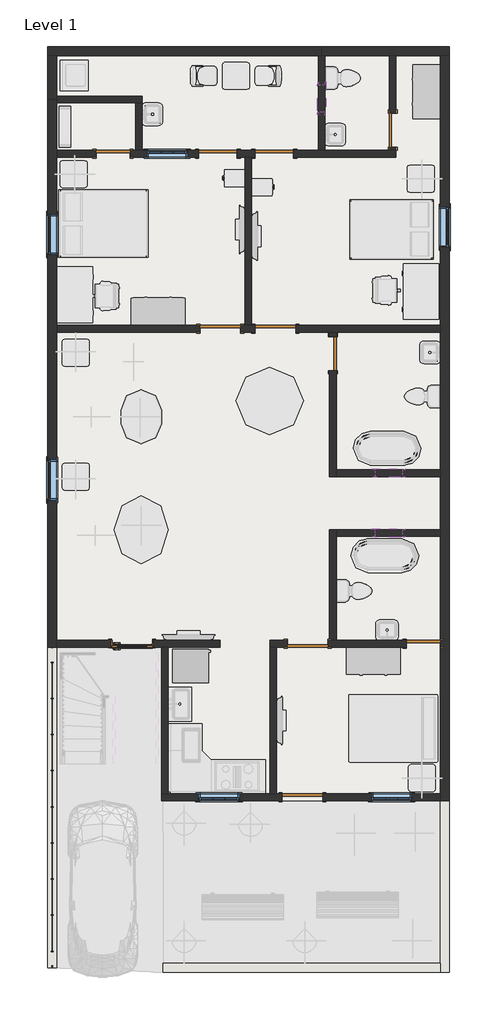
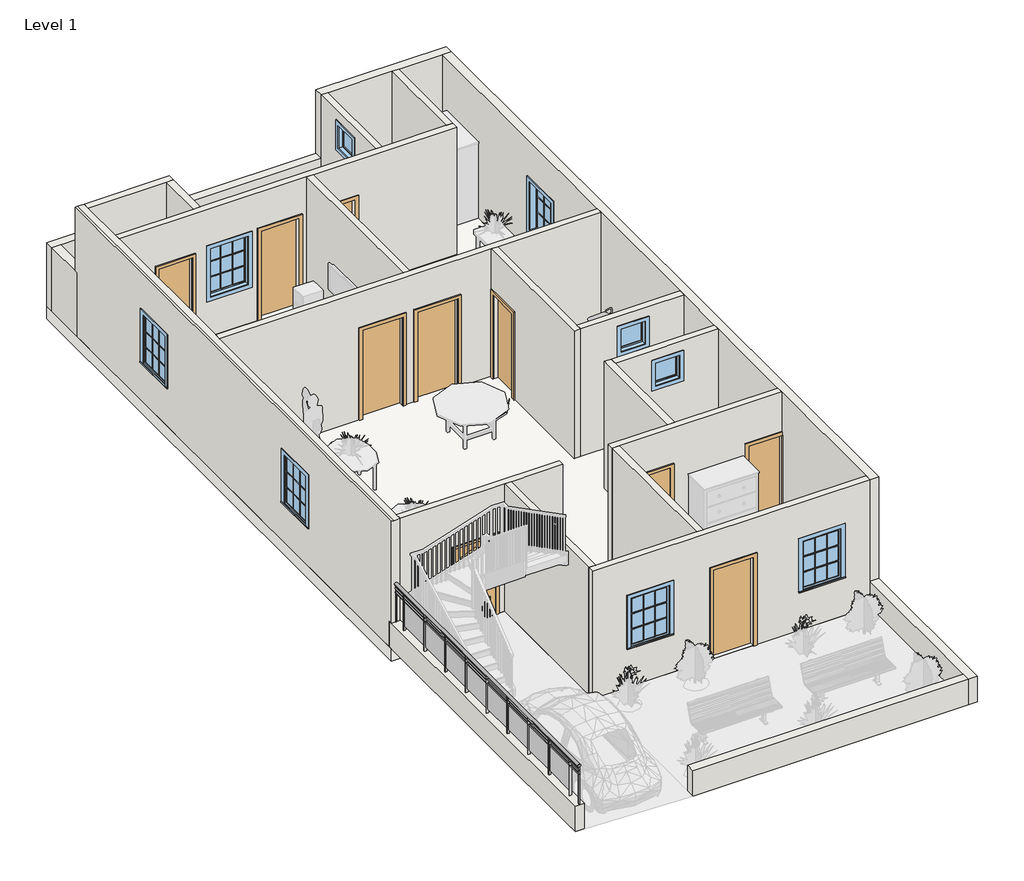
# One storey, part 1 of 3: 24 walls, 11 doors, 9 windows, 1 railing, 1 slab.
"""IFC4 building model written with IfcOpenShell, lengths in millimetres."""

from ifc_helpers import new_model, si_unit, point, frame, origin, origin_with_axes, place, context, project, spatial, polyline, ellipse_curve, trimmed, outline, extrude, faceted_brep, transform, mapped, element, save
from ifc_brep_helpers import plane_surface, extruded_surface, advanced_brep
from components import door_6e7732ad, door_059fdd7e, door_255cab33, door_b6e9fca3, door_99d96fc5, door_16372e1c, door_686f89d2, window_5c190c7e, window_29c06734, window_3d781103

model = new_model("IFC4")

# Units and contexts
model_context = context("Model", 3, world=origin())
ifc_project = project(units=[si_unit("LENGTHUNIT", "METRE", prefix="MILLI")], contexts=[model_context])

# Site, building, storey
site = spatial("IfcSite", under=ifc_project)
building = spatial("IfcBuilding", under=site)
storey = spatial("IfcBuildingStorey", under=building, Name="Level 1", Elevation=0.0)

# Doors
placement = place(None, origin())
door_shape = door_6e7732ad(model_context)
element("IfcDoor", 1, ObjectType="36\" x 74\"", at=placement, inside=storey, context=model_context, shape_type="MappedRepresentation", body=[
    mapped(door_shape, transform((-11373.4589543, -1136.727182, 0.0), x_axis=(-1.0, 0.0, 0.0), y_axis=(0.0, -1.0, 0.0), z_axis=(0.0, 0.0, 1.0))),
])
door_2_shape = door_059fdd7e(model_context)
element("IfcDoor", 2, ObjectType="Single-Flush : 30\" x 80\"", at=placement, inside=storey, context=model_context, shape_type="MappedRepresentation", body=[
    mapped(door_2_shape, transform((-11805.2589543, 9890.047818, 0.0), x_axis=(1.0, 0.0, 0.0), y_axis=(0.0, 1.0, 0.0), z_axis=(0.0, 0.0, 1.0))),
])
element("IfcDoor", 3, ObjectType="Single-Flush : 30\" x 80\"", at=placement, inside=storey, context=model_context, shape_type="MappedRepresentation", body=[
    mapped(door_2_shape, transform((-4820.2589543, -1133.552182, 0.0), x_axis=(1.0, 0.0, 0.0), y_axis=(0.0, 1.0, 0.0), z_axis=(0.0, 0.0, 1.0))),
])
door_3_shape = door_255cab33(model_context)
element("IfcDoor", 4, ObjectType="Single-Flush : 30\" x 80\"", at=placement, inside=storey, context=model_context, shape_type="MappedRepresentation", body=[
    mapped(door_3_shape, transform((-5506.0589543, 10423.447818, 0.0), x_axis=(0.0, -1.0, 0.0), y_axis=(1.0, 0.0, 0.0), z_axis=(0.0, 0.0, 1.0))),
])
element("IfcDoor", 5, ObjectType="Single-Flush : 30\" x 80\"", at=placement, inside=storey, context=model_context, shape_type="MappedRepresentation", body=[
    mapped(door_3_shape, transform((-6852.2589543, 5394.247818, 0.0), x_axis=(0.0, 1.0, 0.0), y_axis=(-1.0, 0.0, 0.0), z_axis=(0.0, 0.0, 1.0))),
])
door_4_shape = door_b6e9fca3(model_context)
element("IfcDoor", 6, ObjectType="Single-Flush : 34\" x 84\"", at=placement, inside=storey, context=model_context, shape_type="MappedRepresentation", body=[
    mapped(door_4_shape, transform((-9443.0589543, 9890.047818, 0.0), x_axis=(1.0, 0.0, 0.0), y_axis=(0.0, 1.0, 0.0), z_axis=(0.0, 0.0, 1.0))),
])
door_5_shape = door_99d96fc5(model_context)
element("IfcDoor", 7, ObjectType="Single-Flush : 34\" x 84\"", at=placement, inside=storey, context=model_context, shape_type="MappedRepresentation", body=[
    mapped(door_5_shape, transform((-8173.0589543, 9890.047818, 0.0), x_axis=(-1.0, 0.0, 0.0), y_axis=(0.0, -1.0, 0.0), z_axis=(0.0, 0.0, 1.0))),
])
door_6_shape = door_16372e1c(model_context)
element("IfcDoor", 8, ObjectType="Single-Flush : 36\" x 84\"", at=placement, inside=storey, context=model_context, shape_type="MappedRepresentation", body=[
    mapped(door_6_shape, transform((-9392.2589543, 5953.047818, 0.0), x_axis=(1.0, 0.0, 0.0), y_axis=(0.0, 1.0, 0.0), z_axis=(0.0, 0.0, 1.0))),
])
element("IfcDoor", 9, ObjectType="Single-Flush : 36\" x 84\"", at=placement, inside=storey, context=model_context, shape_type="MappedRepresentation", body=[
    mapped(door_6_shape, transform((-7423.7589543, -1133.552182, 0.0), x_axis=(-1.0, 0.0, 0.0), y_axis=(0.0, -1.0, 0.0), z_axis=(0.0, 0.0, 1.0))),
])
door_7_shape = door_686f89d2(model_context)
element("IfcDoor", 10, ObjectType="Single-Flush : 36\" x 84\"", at=placement, inside=storey, context=model_context, shape_type="MappedRepresentation", body=[
    mapped(door_7_shape, transform((-8147.6589543, 5953.047818, 0.0), x_axis=(-1.0, 0.0, 0.0), y_axis=(0.0, -1.0, 0.0), z_axis=(0.0, 0.0, 1.0))),
])
element("IfcDoor", 11, ObjectType="Single-Flush : 36\" x 84\"", at=placement, inside=storey, context=model_context, shape_type="MappedRepresentation", body=[
    mapped(door_7_shape, transform((-7538.0589543, -4587.952182, 0.0), x_axis=(-1.0, 0.0, 0.0), y_axis=(0.0, -1.0, 0.0), z_axis=(0.0, 0.0, 1.0))),
])

# Railing
element("IfcRailing", 12, ObjectType="Glass Panel - Bottom Fill", at=placement, inside=storey, context=model_context, shape_type="SolidModel", body=[
    advanced_brep(
    [(-13138.7589543, -1209.752182, 1524.0), (-13214.9589543, -1209.752182, 1524.0), (-13138.7589543, -8397.952182, 1524.0), (-13214.9589543, -8397.952182, 1524.0)],
    [
        (0, 1, ellipse_curve(frame((-13176.8589543, -1209.752182, 1524.0), z_axis=(0.0, 1.0, 0.0), x_axis=(-1.0, 0.0, 0.0)), 38.1, 28.575)),
        (1, 0, ellipse_curve(frame((-13176.8589543, -1209.752182, 1524.0), z_axis=(0.0, 1.0, 0.0), x_axis=(-1.0, 0.0, 0.0)), 38.1, 28.575)),
        (2, 3, ellipse_curve(frame((-13176.8589543, -8397.952182, 1524.0), z_axis=(0.0, -1.0, 0.0), x_axis=(-1.0, 0.0, 0.0)), 38.1, 28.575)),
        (3, 2, ellipse_curve(frame((-13176.8589543, -8397.952182, 1524.0), z_axis=(0.0, -1.0, 0.0), x_axis=(-1.0, 0.0, 0.0)), 38.1, 28.575)),
        (0, 2),
        (3, 1),
    ],
    [
        plane_surface(frame((-13176.8589543, -1209.752182, 1524.0), z_axis=(0.0, 1.0, 0.0), x_axis=(0.0, 0.0, -1.0))),
        plane_surface(frame((-13176.8589543, -8397.952182, 1524.0), z_axis=(0.0, -1.0, 0.0), x_axis=(0.0, 0.0, -1.0))),
        extruded_surface(trimmed(ellipse_curve(frame((-13176.8589543, -8397.952182, 1524.0), z_axis=(0.0, 1.0, 0.0), x_axis=(-1.0, 0.0, 0.0)), 38.1, 28.575), [point((-13138.7589543, -8397.952182, 1524.0))], [point((-13214.9589543, -8397.952182, 1524.0))], True, "CARTESIAN"), (0.0, 7188.200000000001, 0.0), 7188.200000000001),
        extruded_surface(trimmed(ellipse_curve(frame((-13176.8589543, -8397.952182, 1524.0), z_axis=(0.0, 1.0, 0.0), x_axis=(-1.0, 0.0, 0.0)), 38.1, 28.575), [point((-13214.9589543, -8397.952182, 1524.0))], [point((-13138.7589543, -8397.952182, 1524.0))], True, "CARTESIAN"), (0.0, 7188.200000000001, 0.0), 7188.200000000001),
    ],
    [
        (0, [[1, 2]]),
        (1, [[3, 4]]),
        (2, [[-1, 5, -4, 6]]),
        (3, [[-2, -6, -3, -5]]),
    ],
),
    extrude(outline(polyline([(-13189.5589543, -1209.752182), (-13164.1589543, -1209.752182), (-13164.1589543, -8397.952182), (-13189.5589543, -8397.952182), (-13189.5589543, -1209.752182)])), frame((0.0, 0.0, 1409.7), z_axis=(0.0, 0.0, 1.0), x_axis=(1.0, 0.0, 0.0)), (0.0, 0.0, 1.0), 25.4),
    extrude(outline(polyline([(-13189.5589543, -1209.752182), (-13164.1589543, -1209.752182), (-13164.1589543, -8397.952182), (-13189.5589543, -8397.952182), (-13189.5589543, -1209.752182)])), frame((0.0, 0.0, 1308.1), z_axis=(0.0, 0.0, 1.0), x_axis=(1.0, 0.0, 0.0)), (0.0, 0.0, 1.0), 25.4),
    extrude(outline(polyline([(-13202.2589543, -8048.702182), (-13151.4589543, -8048.702182), (-13151.4589543, -8061.402182), (-13202.2589543, -8061.402182), (-13202.2589543, -8048.702182)])), frame((0.0, 0.0, 609.6), z_axis=(0.0, 0.0, 1.0), x_axis=(1.0, 0.0, 0.0)), (0.0, 0.0, 1.0), 885.6788223),
    extrude(outline(polyline([(-13170.3237973, -7242.252182), (-13170.3237973, -8055.052182), (-13176.6737973, -8055.052182), (-13176.6737973, -7242.252182), (-13170.3237973, -7242.252182)])), frame((0.0, 0.0, 711.2), z_axis=(0.0, 0.0, 1.0), x_axis=(1.0, 0.0, 0.0)), (0.0, 0.0, 1.0), 596.9),
    extrude(outline(polyline([(-13202.2589543, -7235.902182), (-13151.4589543, -7235.902182), (-13151.4589543, -7248.602182), (-13202.2589543, -7248.602182), (-13202.2589543, -7235.902182)])), frame((0.0, 0.0, 609.6), z_axis=(0.0, 0.0, 1.0), x_axis=(1.0, 0.0, 0.0)), (0.0, 0.0, 1.0), 885.6788223),
    extrude(outline(polyline([(-13170.3237973, -6429.452182), (-13170.3237973, -7242.252182), (-13176.6737973, -7242.252182), (-13176.6737973, -6429.452182), (-13170.3237973, -6429.452182)])), frame((0.0, 0.0, 711.2), z_axis=(0.0, 0.0, 1.0), x_axis=(1.0, 0.0, 0.0)), (0.0, 0.0, 1.0), 596.9),
    extrude(outline(polyline([(-13202.2589543, -6423.102182), (-13151.4589543, -6423.102182), (-13151.4589543, -6435.802182), (-13202.2589543, -6435.802182), (-13202.2589543, -6423.102182)])), frame((0.0, 0.0, 609.6), z_axis=(0.0, 0.0, 1.0), x_axis=(1.0, 0.0, 0.0)), (0.0, 0.0, 1.0), 885.6788223),
    extrude(outline(polyline([(-13170.3237973, -5616.652182), (-13170.3237973, -6429.452182), (-13176.6737973, -6429.452182), (-13176.6737973, -5616.652182), (-13170.3237973, -5616.652182)])), frame((0.0, 0.0, 711.2), z_axis=(0.0, 0.0, 1.0), x_axis=(1.0, 0.0, 0.0)), (0.0, 0.0, 1.0), 596.9),
    extrude(outline(polyline([(-13202.2589543, -5610.302182), (-13151.4589543, -5610.302182), (-13151.4589543, -5623.002182), (-13202.2589543, -5623.002182), (-13202.2589543, -5610.302182)])), frame((0.0, 0.0, 609.6), z_axis=(0.0, 0.0, 1.0), x_axis=(1.0, 0.0, 0.0)), (0.0, 0.0, 1.0), 885.6788223),
    extrude(outline(polyline([(-13170.3237973, -4803.852182), (-13170.3237973, -5616.652182), (-13176.6737973, -5616.652182), (-13176.6737973, -4803.852182), (-13170.3237973, -4803.852182)])), frame((0.0, 0.0, 711.2), z_axis=(0.0, 0.0, 1.0), x_axis=(1.0, 0.0, 0.0)), (0.0, 0.0, 1.0), 596.9),
    extrude(outline(polyline([(-13202.2589543, -4797.502182), (-13151.4589543, -4797.502182), (-13151.4589543, -4810.202182), (-13202.2589543, -4810.202182), (-13202.2589543, -4797.502182)])), frame((0.0, 0.0, 609.6), z_axis=(0.0, 0.0, 1.0), x_axis=(1.0, 0.0, 0.0)), (0.0, 0.0, 1.0), 885.6788223),
    extrude(outline(polyline([(-13170.3237973, -3991.052182), (-13170.3237973, -4803.852182), (-13176.6737973, -4803.852182), (-13176.6737973, -3991.052182), (-13170.3237973, -3991.052182)])), frame((0.0, 0.0, 711.2), z_axis=(0.0, 0.0, 1.0), x_axis=(1.0, 0.0, 0.0)), (0.0, 0.0, 1.0), 596.9),
    extrude(outline(polyline([(-13202.2589543, -3984.702182), (-13151.4589543, -3984.702182), (-13151.4589543, -3997.402182), (-13202.2589543, -3997.402182), (-13202.2589543, -3984.702182)])), frame((0.0, 0.0, 609.6), z_axis=(0.0, 0.0, 1.0), x_axis=(1.0, 0.0, 0.0)), (0.0, 0.0, 1.0), 885.6788223),
    extrude(outline(polyline([(-13170.3237973, -3178.252182), (-13170.3237973, -3991.052182), (-13176.6737973, -3991.052182), (-13176.6737973, -3178.252182), (-13170.3237973, -3178.252182)])), frame((0.0, 0.0, 711.2), z_axis=(0.0, 0.0, 1.0), x_axis=(1.0, 0.0, 0.0)), (0.0, 0.0, 1.0), 596.9),
    extrude(outline(polyline([(-13202.2589543, -3171.902182), (-13151.4589543, -3171.902182), (-13151.4589543, -3184.602182), (-13202.2589543, -3184.602182), (-13202.2589543, -3171.902182)])), frame((0.0, 0.0, 609.6), z_axis=(0.0, 0.0, 1.0), x_axis=(1.0, 0.0, 0.0)), (0.0, 0.0, 1.0), 885.6788223),
    extrude(outline(polyline([(-13170.3237973, -2365.452182), (-13170.3237973, -3178.252182), (-13176.6737973, -3178.252182), (-13176.6737973, -2365.452182), (-13170.3237973, -2365.452182)])), frame((0.0, 0.0, 711.2), z_axis=(0.0, 0.0, 1.0), x_axis=(1.0, 0.0, 0.0)), (0.0, 0.0, 1.0), 596.9),
    extrude(outline(polyline([(-13202.2589543, -2359.102182), (-13151.4589543, -2359.102182), (-13151.4589543, -2371.802182), (-13202.2589543, -2371.802182), (-13202.2589543, -2359.102182)])), frame((0.0, 0.0, 609.6), z_axis=(0.0, 0.0, 1.0), x_axis=(1.0, 0.0, 0.0)), (0.0, 0.0, 1.0), 885.6788223),
    extrude(outline(polyline([(-13170.3237973, -1552.652182), (-13170.3237973, -2365.452182), (-13176.6737973, -2365.452182), (-13176.6737973, -1552.652182), (-13170.3237973, -1552.652182)])), frame((0.0, 0.0, 711.2), z_axis=(0.0, 0.0, 1.0), x_axis=(1.0, 0.0, 0.0)), (0.0, 0.0, 1.0), 596.9),
    extrude(outline(polyline([(-13202.2589543, -1546.302182), (-13151.4589543, -1546.302182), (-13151.4589543, -1559.002182), (-13202.2589543, -1559.002182), (-13202.2589543, -1546.302182)])), frame((0.0, 0.0, 609.6), z_axis=(0.0, 0.0, 1.0), x_axis=(1.0, 0.0, 0.0)), (0.0, 0.0, 1.0), 885.6788223),
    extrude(outline(polyline([(-13186.3839543, -8385.252182), (-13167.3339543, -8385.252182), (-13167.3339543, -8404.302182), (-13186.3839543, -8404.302182), (-13186.3839543, -8385.252182)])), frame((0.0, 0.0, 609.6), z_axis=(0.0, 0.0, 1.0), x_axis=(1.0, 0.0, 0.0)), (0.0, 0.0, 1.0), 885.6788223),
    extrude(outline(polyline([(-13186.3839543, -1203.402182), (-13167.3339543, -1203.402182), (-13167.3339543, -1222.452182), (-13186.3839543, -1222.452182), (-13186.3839543, -1203.402182)])), frame((0.0, 0.0, 609.6), z_axis=(0.0, 0.0, 1.0), x_axis=(1.0, 0.0, 0.0)), (0.0, 0.0, 1.0), 885.6788223),
])

# Slab
element("IfcSlab", 13, ObjectType="Generic - 12\"", at=placement, inside=storey, context=model_context, shape_type="SweptSolid", body=[
    extrude(outline(polyline([(-4236.0589543, 12303.047818), (-4236.0589543, -4664.152182), (-10713.0589543, -4664.152182), (-10713.0589543, -1209.752182), (-13278.4589543, -1209.752182), (-13278.4589543, 12303.047818), (-4236.0589543, 12303.047818)])), frame((0.0, 0.0, -304.8), z_axis=(0.0, 0.0, 1.0), x_axis=(1.0, 0.0, 0.0)), (0.0, 0.0, 1.0), 304.8),
])

# Walls
element("IfcWall", 14, ObjectType="Generic - 2'", at=placement, inside=storey, context=model_context, shape_type="Brep", body=[
    faceted_brep([(-13278.4589543, 12099.847818, 0.0), (-13075.2589543, 12099.847818, 0.0), (-7182.4589543, 12099.847818, 0.0), (-7106.2589543, 12099.847818, 0.0), (-7106.2589543, 12099.847818, 1524.0), (-13075.2589543, 12099.847818, 1524.0), (-13278.4589543, 12099.847818, 1524.0), (-13278.4589543, 12303.047818, 0.0), (-13278.4589543, 12303.047818, 1524.0), (-7106.2589543, 12303.047818, 1524.0), (-7106.2589543, 12303.047818, 0.0)], [[[0, 1, 2, 3, 4, 5, 6]], [[7, 8, 9, 10]], [[3, 2, 1, 0, 7, 10]], [[4, 3, 10, 9]], [[6, 5, 4, 9, 8]], [[0, 6, 8, 7]]]),
])
element("IfcWall", 15, ObjectType="Generic - 2'", at=placement, inside=storey, context=model_context, shape_type="SweptSolid", body=[
    extrude(outline(polyline([(-10674.9589543, -8321.752182), (-4439.2589543, -8321.752182), (-4439.2589543, -8524.952182), (-10674.9589543, -8524.952182), (-10674.9589543, -8321.752182)])), origin_with_axes(), (0.0, 0.0, 1.0), 609.6),
])
element("IfcWall", 16, ObjectType="Generic - 2'", at=placement, inside=storey, context=model_context, shape_type="Brep", body=[
    faceted_brep([(-13075.2589543, -8423.352182, 0.0), (-13075.2589543, -1209.752182, 0.0), (-13075.2589543, -1133.552182, 0.0), (-13075.2589543, -1133.552182, 609.6), (-13075.2589543, -8423.352182, 609.6), (-13278.4589543, -8423.352182, 0.0), (-13278.4589543, -8423.352182, 609.6), (-13278.4589543, -1133.552182, 609.6), (-13278.4589543, -1133.552182, 0.0)], [[[0, 1, 2, 3, 4]], [[5, 6, 7, 8]], [[2, 1, 0, 5, 8]], [[3, 2, 8, 7]], [[4, 3, 7, 6]], [[0, 4, 6, 5]]]),
])
element("IfcWall", 17, ObjectType="Generic - 2'", at=placement, inside=storey, context=model_context, shape_type="Brep", body=[
    faceted_brep([(-13075.2589543, 11109.247818, 0.0), (-13075.2589543, 11185.447818, 0.0), (-13075.2589543, 12099.847818, 0.0), (-13075.2589543, 12099.847818, 1524.0), (-13075.2589543, 11109.247818, 1524.0), (-13278.4589543, 11109.247818, 0.0), (-13278.4589543, 11109.247818, 1524.0), (-13278.4589543, 12099.847818, 1524.0), (-13278.4589543, 12099.847818, 0.0)], [[[0, 1, 2, 3, 4]], [[5, 6, 7, 8]], [[2, 1, 0, 5, 8]], [[4, 3, 7, 6]], [[0, 4, 6, 5]], [[3, 2, 8, 7]]]),
])
element("IfcWall", 18, ObjectType="Generic - 2'", at=placement, inside=storey, context=model_context, shape_type="Brep", body=[
    faceted_brep([(-4439.2589543, -4587.952182, 0.0), (-4439.2589543, -4664.152182, 0.0), (-4439.2589543, -8321.752182, 0.0), (-4439.2589543, -8524.952182, 0.0), (-4439.2589543, -8524.952182, 609.6), (-4439.2589543, -8321.752182, 609.6), (-4439.2589543, -4587.952182, 609.6), (-4236.0589543, -4587.952182, 0.0), (-4236.0589543, -4587.952182, 609.6), (-4236.0589543, -8524.952182, 609.6), (-4236.0589543, -8524.952182, 0.0)], [[[0, 1, 2, 3, 4, 5, 6]], [[7, 8, 9, 10]], [[3, 2, 1, 0, 7, 10]], [[6, 5, 4, 9, 8]], [[0, 6, 8, 7]], [[4, 3, 10, 9]]]),
])
element("IfcWall", 19, ObjectType="Generic - 8\"", at=placement, inside=storey, context=model_context, shape_type="Brep", body=[
    faceted_brep([(-4439.2589543, 12099.847818, 0.0), (-4439.2589543, 6029.247818, 0.0), (-4439.2589543, 5876.847818, 0.0), (-4439.2589543, 2778.047818, 0.0), (-4439.2589543, 2625.647818, 0.0), (-4439.2589543, 1431.847818, 0.0), (-4439.2589543, 1279.447818, 0.0), (-4439.2589543, -4511.752182, 0.0), (-4439.2589543, -4587.952182, 0.0), (-4439.2589543, -4587.952182, 609.6), (-4439.2589543, -4664.152182, 609.6), (-4439.2589543, -4664.152182, 3048.0), (-4439.2589543, -4511.752182, 3048.0), (-4439.2589543, -1209.752182, 3048.0), (-4439.2589543, -1057.352182, 3048.0), (-4439.2589543, 1279.447818, 3048.0), (-4439.2589543, 1431.847818, 3048.0), (-4439.2589543, 2625.647818, 3048.0), (-4439.2589543, 2778.047818, 3048.0), (-4439.2589543, 5876.847818, 3048.0), (-4439.2589543, 6029.247818, 3048.0), (-4439.2589543, 12099.847818, 3048.0), (-4439.2589543, 7781.847818, 2133.6), (-4439.2589543, 7781.847818, 914.4), (-4439.2589543, 8696.247818, 914.4), (-4439.2589543, 8696.247818, 2133.6), (-4236.0589543, 12099.847818, 0.0), (-4236.0589543, 12099.847818, 3048.0), (-4236.0589543, -4664.152182, 3048.0), (-4236.0589543, -4664.152182, 609.6), (-4236.0589543, -4587.952182, 609.6), (-4236.0589543, -4587.952182, 0.0), (-4236.0589543, 7781.847818, 2133.6), (-4236.0589543, 8696.247818, 2133.6), (-4236.0589543, 8696.247818, 914.4), (-4236.0589543, 7781.847818, 914.4)], [[[0, 1, 2, 3, 4, 5, 6, 7, 8, 9, 10, 11, 12, 13, 14, 15, 16, 17, 18, 19, 20, 21], [22, 23, 24, 25]], [[26, 27, 28, 29, 30, 31], [32, 33, 34, 35]], [[8, 7, 6, 5, 4, 3, 2, 1, 0, 26, 31]], [[0, 21, 27, 26]], [[23, 22, 32, 35]], [[24, 23, 35, 34]], [[25, 24, 34, 33]], [[22, 25, 33, 32]], [[9, 8, 31, 30]], [[29, 10, 9, 30]], [[11, 10, 29, 28]], [[21, 20, 19, 18, 17, 16, 15, 14, 13, 12, 11, 28, 27]]]),
])
element("IfcWall", 20, ObjectType="Generic - 8\"", at=placement, inside=storey, context=model_context, shape_type="Brep", body=[
    faceted_brep([(-7106.2589543, 12099.847818, 0.0), (-7030.0589543, 12099.847818, 0.0), (-5582.2589543, 12099.847818, 0.0), (-5429.8589543, 12099.847818, 0.0), (-4439.2589543, 12099.847818, 0.0), (-4236.0589543, 12099.847818, 0.0), (-4236.0589543, 12099.847818, 3048.0), (-4439.2589543, 12099.847818, 3048.0), (-5429.8589543, 12099.847818, 3048.0), (-5582.2589543, 12099.847818, 3048.0), (-7030.0589543, 12099.847818, 3048.0), (-7182.4589543, 12099.847818, 3048.0), (-7182.4589543, 12099.847818, 1524.0), (-7106.2589543, 12099.847818, 1524.0), (-7106.2589543, 12303.047818, 0.0), (-7106.2589543, 12303.047818, 1524.0), (-7182.4589543, 12303.047818, 1524.0), (-7182.4589543, 12303.047818, 3048.0), (-4236.0589543, 12303.047818, 3048.0), (-4236.0589543, 12303.047818, 0.0)], [[[0, 1, 2, 3, 4, 5, 6, 7, 8, 9, 10, 11, 12, 13]], [[14, 15, 16, 17, 18, 19]], [[5, 4, 3, 2, 1, 0, 14, 19]], [[6, 5, 19, 18]], [[0, 13, 15, 14]], [[12, 16, 15, 13]], [[12, 11, 17, 16]], [[11, 10, 9, 8, 7, 6, 18, 17]]]),
])
element("IfcWall", 21, ObjectType="Generic - 8\"", at=placement, inside=storey, context=model_context, shape_type="Brep", body=[
    faceted_brep([(-13075.2589543, -1133.552182, 0.0), (-13075.2589543, -1057.352182, 0.0), (-13075.2589543, 5876.847818, 0.0), (-13075.2589543, 6029.247818, 0.0), (-13075.2589543, 9813.847818, 0.0), (-13075.2589543, 9966.247818, 0.0), (-13075.2589543, 11033.047818, 0.0), (-13075.2589543, 11109.247818, 0.0), (-13075.2589543, 11109.247818, 1524.0), (-13075.2589543, 11185.447818, 1524.0), (-13075.2589543, 11185.447818, 3048.0), (-13075.2589543, 11033.047818, 3048.0), (-13075.2589543, 9966.247818, 3048.0), (-13075.2589543, 9813.847818, 3048.0), (-13075.2589543, 6029.247818, 3048.0), (-13075.2589543, 5876.847818, 3048.0), (-13075.2589543, -1057.352182, 3048.0), (-13075.2589543, -1209.752182, 3048.0), (-13075.2589543, -1209.752182, 609.6), (-13075.2589543, -1133.552182, 609.6), (-13075.2589543, 3006.647818, 2133.6), (-13075.2589543, 3006.647818, 914.4), (-13075.2589543, 2092.247818, 914.4), (-13075.2589543, 2092.247818, 2133.6), (-13075.2589543, 8531.147818, 2133.6), (-13075.2589543, 8531.147818, 914.4), (-13075.2589543, 7616.747818, 914.4), (-13075.2589543, 7616.747818, 2133.6), (-13278.4589543, -1133.552182, 0.0), (-13278.4589543, -1133.552182, 609.6), (-13278.4589543, -1209.752182, 609.6), (-13278.4589543, -1209.752182, 3048.0), (-13278.4589543, 11185.447818, 3048.0), (-13278.4589543, 11185.447818, 1524.0), (-13278.4589543, 11109.247818, 1524.0), (-13278.4589543, 11109.247818, 0.0), (-13278.4589543, 3006.647818, 2133.6), (-13278.4589543, 2092.247818, 2133.6), (-13278.4589543, 2092.247818, 914.4), (-13278.4589543, 3006.647818, 914.4), (-13278.4589543, 8531.147818, 2133.6), (-13278.4589543, 7616.747818, 2133.6), (-13278.4589543, 7616.747818, 914.4), (-13278.4589543, 8531.147818, 914.4), (-13227.6589543, 11185.447818, 3048.0), (-13227.6589543, -1209.752182, 3048.0)], [[[0, 1, 2, 3, 4, 5, 6, 7, 8, 9, 10, 11, 12, 13, 14, 15, 16, 17, 18, 19], [20, 21, 22, 23], [24, 25, 26, 27]], [[28, 29, 30, 31, 32, 33, 34, 35], [36, 37, 38, 39], [40, 41, 42, 43]], [[7, 6, 5, 4, 3, 2, 1, 0, 28, 35]], [[8, 7, 35, 34]], [[33, 9, 8, 34]], [[10, 9, 33, 32, 44]], [[20, 23, 37, 36]], [[23, 22, 38, 37]], [[22, 21, 39, 38]], [[21, 20, 36, 39]], [[24, 27, 41, 40]], [[27, 26, 42, 41]], [[26, 25, 43, 42]], [[25, 24, 40, 43]], [[0, 19, 29, 28]], [[18, 30, 29, 19]], [[18, 17, 45, 31, 30]], [[44, 32, 31, 45]], [[17, 16, 15, 14, 13, 12, 11, 10, 44, 45]]]),
])
element("IfcWall", 22, ObjectType="INNER 6\"", at=placement, inside=storey, context=model_context, shape_type="Brep", body=[
    faceted_brep([(-9011.2589543, 9813.847818, 0.0), (-8833.4589543, 9813.847818, 0.0), (-8681.0589543, 9813.847818, 0.0), (-8604.8589543, 9813.847818, 0.0), (-8604.8589543, 9813.847818, 2133.6), (-7741.2589543, 9813.847818, 2133.6), (-7741.2589543, 9813.847818, 0.0), (-5429.8589543, 9813.847818, 0.0), (-5429.8589543, 9813.847818, 3048.0), (-8681.0589543, 9813.847818, 3048.0), (-8833.4589543, 9813.847818, 3048.0), (-13075.2589543, 9813.847818, 3048.0), (-13075.2589543, 9813.847818, 0.0), (-12186.2589543, 9813.847818, 0.0), (-12186.2589543, 9813.847818, 2032.0), (-11424.2589543, 9813.847818, 2032.0), (-11424.2589543, 9813.847818, 0.0), (-9874.8589543, 9813.847818, 0.0), (-9874.8589543, 9813.847818, 2133.6), (-9011.2589543, 9813.847818, 2133.6), (-10128.8589543, 9813.847818, 2133.6), (-10128.8589543, 9813.847818, 914.4), (-11043.2589543, 9813.847818, 914.4), (-11043.2589543, 9813.847818, 2133.6), (-8604.8589543, 9966.247818, 2133.6), (-8604.8589543, 9966.247818, 0.0), (-9011.2589543, 9966.247818, 0.0), (-9011.2589543, 9966.247818, 2133.6), (-9874.8589543, 9966.247818, 2133.6), (-9874.8589543, 9966.247818, 0.0), (-11144.8589543, 9966.247818, 0.0), (-11297.2589543, 9966.247818, 0.0), (-11424.2589543, 9966.247818, 0.0), (-11424.2589543, 9966.247818, 2032.0), (-12186.2589543, 9966.247818, 2032.0), (-12186.2589543, 9966.247818, 0.0), (-13075.2589543, 9966.247818, 0.0), (-13075.2589543, 9966.247818, 3048.0), (-11297.2589543, 9966.247818, 3048.0), (-11144.8589543, 9966.247818, 3048.0), (-7182.4589543, 9966.247818, 3048.0), (-7030.0589543, 9966.247818, 3048.0), (-5582.2589543, 9966.247818, 3048.0), (-5429.8589543, 9966.247818, 3048.0), (-5429.8589543, 9966.247818, 0.0), (-5582.2589543, 9966.247818, 0.0), (-7030.0589543, 9966.247818, 0.0), (-7182.4589543, 9966.247818, 0.0), (-7741.2589543, 9966.247818, 0.0), (-7741.2589543, 9966.247818, 2133.6), (-10128.8589543, 9966.247818, 2133.6), (-11043.2589543, 9966.247818, 2133.6), (-11043.2589543, 9966.247818, 914.4), (-10128.8589543, 9966.247818, 914.4)], [[[0, 1, 2, 3, 4, 5, 6, 7, 8, 9, 10, 11, 12, 13, 14, 15, 16, 17, 18, 19], [20, 21, 22, 23]], [[24, 25, 26, 27, 28, 29, 30, 31, 32, 33, 34, 35, 36, 37, 38, 39, 40, 41, 42, 43, 44, 45, 46, 47, 48, 49], [50, 51, 52, 53]], [[13, 12, 36, 35]], [[17, 16, 32, 31, 30, 29]], [[26, 25, 3, 2, 1, 0]], [[48, 47, 46, 45, 44, 7, 6]], [[12, 11, 37, 36]], [[33, 32, 16, 15]], [[34, 33, 15, 14]], [[35, 34, 14, 13]], [[27, 26, 0, 19]], [[28, 27, 19, 18]], [[29, 28, 18, 17]], [[4, 3, 25, 24]], [[5, 4, 24, 49]], [[6, 5, 49, 48]], [[8, 7, 44, 43]], [[21, 20, 50, 53]], [[22, 21, 53, 52]], [[23, 22, 52, 51]], [[20, 23, 51, 50]], [[11, 10, 9, 8, 43, 42, 41, 40, 39, 38, 37]]]),
])
element("IfcWall", 23, ObjectType="INNER 6\"", at=placement, inside=storey, context=model_context, shape_type="Brep", body=[
    faceted_brep([(-13075.2589543, 11033.047818, 3048.0), (-13075.2589543, 11033.047818, 0.0), (-11297.2589543, 11033.047818, 0.0), (-11144.8589543, 11033.047818, 0.0), (-11144.8589543, 11033.047818, 3048.0), (-11297.2589543, 11033.047818, 3048.0), (-13075.2589543, 11185.447818, 0.0), (-13075.2589543, 11185.447818, 1524.0), (-13075.2589543, 11185.447818, 3048.0), (-11144.8589543, 11185.447818, 3048.0), (-11144.8589543, 11185.447818, 0.0), (-13075.2589543, 11109.247818, 0.0)], [[[0, 1, 2, 3, 4, 5]], [[6, 7, 8, 9, 10]], [[3, 2, 1, 11, 6, 10]], [[4, 3, 10, 9]], [[0, 8, 7, 6, 11, 1]], [[0, 5, 4, 9, 8]]]),
])
element("IfcWall", 24, ObjectType="INNER 6\"", at=placement, inside=storey, context=model_context, shape_type="SweptSolid", body=[
    extrude(outline(polyline([(-11297.2589543, 9966.247818), (-11297.2589543, 11033.047818), (-11144.8589543, 11033.047818), (-11144.8589543, 9966.247818), (-11297.2589543, 9966.247818)])), origin_with_axes(), (0.0, 0.0, 1.0), 3048.0),
])
element("IfcWall", 25, ObjectType="INNER 6\"", at=placement, inside=storey, context=model_context, shape_type="Brep", body=[
    faceted_brep([(-7182.4589543, 12099.847818, 3048.0), (-7182.4589543, 12099.847818, 1524.0), (-7182.4589543, 12099.847818, 0.0), (-7182.4589543, 9966.247818, 0.0), (-7182.4589543, 9966.247818, 3048.0), (-7182.4589543, 10829.847818, 2768.6), (-7182.4589543, 10829.847818, 2159.0), (-7182.4589543, 11439.447818, 2159.0), (-7182.4589543, 11439.447818, 2768.6), (-7030.0589543, 12099.847818, 0.0), (-7030.0589543, 12099.847818, 3048.0), (-7030.0589543, 9966.247818, 3048.0), (-7030.0589543, 9966.247818, 0.0), (-7030.0589543, 10829.847818, 2768.6), (-7030.0589543, 11439.447818, 2768.6), (-7030.0589543, 11439.447818, 2159.0), (-7030.0589543, 10829.847818, 2159.0), (-7106.2589543, 12099.847818, 0.0)], [[[0, 1, 2, 3, 4], [5, 6, 7, 8]], [[9, 10, 11, 12], [13, 14, 15, 16]], [[3, 2, 17, 9, 12]], [[4, 3, 12, 11]], [[6, 5, 13, 16]], [[7, 6, 16, 15]], [[8, 7, 15, 14]], [[5, 8, 14, 13]], [[0, 10, 9, 17, 2, 1]], [[0, 4, 11, 10]]]),
])
element("IfcWall", 26, ObjectType="INNER 6\"", at=placement, inside=storey, context=model_context, shape_type="SweptSolid", body=[
    extrude(outline(polyline([(10042.447818, 2032.0), (10042.447818, 0.0), (9966.247818, 0.0), (9966.247818, 3048.0), (12099.847818, 3048.0), (12099.847818, 0.0), (10804.447818, 0.0), (10804.447818, 2032.0), (10042.447818, 2032.0)])), frame((-5582.2589543, 0.0, 0.0), z_axis=(1.0, 0.0, 0.0), x_axis=(0.0, 1.0, 0.0)), (0.0, 0.0, 1.0), 152.4),
])
element("IfcWall", 27, ObjectType="INNER 6\"", at=placement, inside=storey, context=model_context, shape_type="SweptSolid", body=[
    extrude(outline(polyline([(-8833.4589543, 6029.247818), (-8833.4589543, 9813.847818), (-8681.0589543, 9813.847818), (-8681.0589543, 6029.247818), (-8833.4589543, 6029.247818)])), origin_with_axes(), (0.0, 0.0, 1.0), 3048.0),
])
element("IfcWall", 28, ObjectType="INNER 6\"", at=placement, inside=storey, context=model_context, shape_type="Brep", body=[
    faceted_brep([(-8604.8589543, 6029.247818, 2133.6), (-8604.8589543, 6029.247818, 0.0), (-8681.0589543, 6029.247818, 0.0), (-8833.4589543, 6029.247818, 0.0), (-8935.0589543, 6029.247818, 0.0), (-8935.0589543, 6029.247818, 2133.6), (-9849.4589543, 6029.247818, 2133.6), (-9849.4589543, 6029.247818, 0.0), (-13075.2589543, 6029.247818, 0.0), (-13075.2589543, 6029.247818, 3048.0), (-8833.4589543, 6029.247818, 3048.0), (-8681.0589543, 6029.247818, 3048.0), (-4439.2589543, 6029.247818, 3048.0), (-4439.2589543, 6029.247818, 0.0), (-7690.4589543, 6029.247818, 0.0), (-7690.4589543, 6029.247818, 2133.6), (-8935.0589543, 5876.847818, 0.0), (-8604.8589543, 5876.847818, 0.0), (-8604.8589543, 5876.847818, 2133.6), (-7690.4589543, 5876.847818, 2133.6), (-7690.4589543, 5876.847818, 0.0), (-6928.4589543, 5876.847818, 0.0), (-6776.0589543, 5876.847818, 0.0), (-4439.2589543, 5876.847818, 0.0), (-4439.2589543, 5876.847818, 3048.0), (-6776.0589543, 5876.847818, 3048.0), (-6928.4589543, 5876.847818, 3048.0), (-13075.2589543, 5876.847818, 3048.0), (-13075.2589543, 5876.847818, 0.0), (-9849.4589543, 5876.847818, 0.0), (-9849.4589543, 5876.847818, 2133.6), (-8935.0589543, 5876.847818, 2133.6)], [[[0, 1, 2, 3, 4, 5, 6, 7, 8, 9, 10, 11, 12, 13, 14, 15]], [[16, 17, 18, 19, 20, 21, 22, 23, 24, 25, 26, 27, 28, 29, 30, 31]], [[29, 28, 8, 7]], [[14, 13, 23, 22, 21, 20]], [[4, 3, 2, 1, 17, 16]], [[9, 8, 28, 27]], [[13, 12, 24, 23]], [[5, 4, 16, 31]], [[6, 5, 31, 30]], [[7, 6, 30, 29]], [[18, 17, 1, 0]], [[19, 18, 0, 15]], [[20, 19, 15, 14]], [[12, 11, 10, 9, 27, 26, 25, 24]]]),
])
element("IfcWall", 29, ObjectType="INNER 6\"", at=placement, inside=storey, context=model_context, shape_type="Brep", body=[
    faceted_brep([(-6928.4589543, 5876.847818, 0.0), (-6928.4589543, 5775.247818, 0.0), (-6928.4589543, 5775.247818, 2032.0), (-6928.4589543, 5013.247818, 2032.0), (-6928.4589543, 5013.247818, 0.0), (-6928.4589543, 2625.647818, 0.0), (-6928.4589543, 2625.647818, 3048.0), (-6928.4589543, 5876.847818, 3048.0), (-6776.0589543, 5775.247818, 2032.0), (-6776.0589543, 5775.247818, 0.0), (-6776.0589543, 5876.847818, 0.0), (-6776.0589543, 5876.847818, 3048.0), (-6776.0589543, 2778.047818, 3048.0), (-6776.0589543, 2625.647818, 3048.0), (-6776.0589543, 2625.647818, 0.0), (-6776.0589543, 2778.047818, 0.0), (-6776.0589543, 5013.247818, 0.0), (-6776.0589543, 5013.247818, 2032.0)], [[[0, 1, 2, 3, 4, 5, 6, 7]], [[8, 9, 10, 11, 12, 13, 14, 15, 16, 17]], [[10, 9, 1, 0]], [[16, 15, 14, 5, 4]], [[0, 7, 11, 10]], [[2, 1, 9, 8]], [[3, 2, 8, 17]], [[4, 3, 17, 16]], [[6, 5, 14, 13]], [[7, 6, 13, 12, 11]]]),
])
element("IfcWall", 30, ObjectType="INNER 6\"", at=placement, inside=storey, context=model_context, shape_type="SweptSolid", body=[
    extrude(outline(polyline([(0.0, -6776.0589543), (0.0, -4439.2589543), (3048.0, -4439.2589543), (3048.0, -6776.0589543), (0.0, -6776.0589543)]), holes=[polyline([(2768.6, -5290.1589543), (2159.0, -5290.1589543), (2159.0, -5899.7589543), (2768.6, -5899.7589543), (2768.6, -5290.1589543)])]), frame((0.0, 2625.647818, 0.0), z_axis=(0.0, 1.0, 0.0), x_axis=(0.0, 0.0, 1.0)), (0.0, 0.0, 1.0), 152.4),
])
element("IfcWall", 31, ObjectType="INNER 6\"", at=placement, inside=storey, context=model_context, shape_type="SweptSolid", body=[
    extrude(outline(polyline([(0.0, -6776.0589543), (0.0, -4439.2589543), (3048.0, -4439.2589543), (3048.0, -6776.0589543), (0.0, -6776.0589543)]), holes=[polyline([(2768.6, -5290.1589543), (2159.0, -5290.1589543), (2159.0, -5899.7589543), (2768.6, -5899.7589543), (2768.6, -5290.1589543)])]), frame((0.0, 1279.447818, 0.0), z_axis=(0.0, 1.0, 0.0), x_axis=(0.0, 0.0, 1.0)), (0.0, 0.0, 1.0), 152.4),
])
element("IfcWall", 32, ObjectType="INNER 6\"", at=placement, inside=storey, context=model_context, shape_type="Brep", body=[
    faceted_brep([(-7880.9589543, -1057.352182, 2133.6), (-7880.9589543, -1057.352182, 0.0), (-8274.6589543, -1057.352182, 0.0), (-8274.6589543, -1057.352182, 3048.0), (-6928.4589543, -1057.352182, 3048.0), (-6776.0589543, -1057.352182, 3048.0), (-4439.2589543, -1057.352182, 3048.0), (-4439.2589543, -1057.352182, 2032.0), (-5201.2589543, -1057.352182, 2032.0), (-5201.2589543, -1057.352182, 0.0), (-6776.0589543, -1057.352182, 0.0), (-6928.4589543, -1057.352182, 0.0), (-6966.5589543, -1057.352182, 0.0), (-6966.5589543, -1057.352182, 2133.6), (-8274.6589543, -1209.752182, 0.0), (-8122.2589543, -1209.752182, 0.0), (-7880.9589543, -1209.752182, 0.0), (-7880.9589543, -1209.752182, 2133.6), (-6966.5589543, -1209.752182, 2133.6), (-6966.5589543, -1209.752182, 0.0), (-5201.2589543, -1209.752182, 0.0), (-5201.2589543, -1209.752182, 2032.0), (-4439.2589543, -1209.752182, 2032.0), (-4439.2589543, -1209.752182, 3048.0), (-8122.2589543, -1209.752182, 3048.0), (-8274.6589543, -1209.752182, 3048.0)], [[[0, 1, 2, 3, 4, 5, 6, 7, 8, 9, 10, 11, 12, 13]], [[14, 15, 16, 17, 18, 19, 20, 21, 22, 23, 24, 25]], [[2, 1, 16, 15, 14]], [[12, 11, 10, 9, 20, 19]], [[6, 23, 22, 7]], [[17, 16, 1, 0]], [[18, 17, 0, 13]], [[19, 18, 13, 12]], [[21, 8, 7, 22]], [[8, 21, 20, 9]], [[3, 2, 14, 25]], [[6, 5, 4, 3, 25, 24, 23]]]),
])
element("IfcWall", 33, ObjectType="INNER 6\"", at=placement, inside=storey, context=model_context, shape_type="SweptSolid", body=[
    extrude(outline(polyline([(-8274.6589543, -4511.752182), (-8274.6589543, -1209.752182), (-8122.2589543, -1209.752182), (-8122.2589543, -4511.752182), (-8274.6589543, -4511.752182)])), origin_with_axes(), (0.0, 0.0, 1.0), 3048.0),
])
element("IfcWall", 34, ObjectType="INNER 6\"", at=placement, inside=storey, context=model_context, shape_type="Brep", body=[
    faceted_brep([(-10713.0589543, -4664.152182, 0.0), (-7995.2589543, -4664.152182, 0.0), (-7995.2589543, -4664.152182, 2133.6), (-7080.8589543, -4664.152182, 2133.6), (-7080.8589543, -4664.152182, 0.0), (-4439.2589543, -4664.152182, 0.0), (-4439.2589543, -4664.152182, 609.6), (-4439.2589543, -4664.152182, 3048.0), (-10713.0589543, -4664.152182, 3048.0), (-5988.6589543, -4664.152182, 2133.6), (-5074.2589543, -4664.152182, 2133.6), (-5074.2589543, -4664.152182, 914.4), (-5988.6589543, -4664.152182, 914.4), (-9874.8589543, -4664.152182, 2133.6), (-8960.4589543, -4664.152182, 2133.6), (-8960.4589543, -4664.152182, 914.4), (-9874.8589543, -4664.152182, 914.4), (-7995.2589543, -4511.752182, 2133.6), (-7995.2589543, -4511.752182, 0.0), (-8122.2589543, -4511.752182, 0.0), (-8274.6589543, -4511.752182, 0.0), (-10560.6589543, -4511.752182, 0.0), (-10713.0589543, -4511.752182, 0.0), (-10713.0589543, -4511.752182, 3048.0), (-10560.6589543, -4511.752182, 3048.0), (-8274.6589543, -4511.752182, 3048.0), (-8122.2589543, -4511.752182, 3048.0), (-4439.2589543, -4511.752182, 3048.0), (-4439.2589543, -4511.752182, 0.0), (-7080.8589543, -4511.752182, 0.0), (-7080.8589543, -4511.752182, 2133.6), (-5988.6589543, -4511.752182, 2133.6), (-5988.6589543, -4511.752182, 914.4), (-5074.2589543, -4511.752182, 914.4), (-5074.2589543, -4511.752182, 2133.6), (-9874.8589543, -4511.752182, 2133.6), (-9874.8589543, -4511.752182, 914.4), (-8960.4589543, -4511.752182, 914.4), (-8960.4589543, -4511.752182, 2133.6), (-4439.2589543, -4587.952182, 0.0)], [[[0, 1, 2, 3, 4, 5, 6, 7, 8], [9, 10, 11, 12], [13, 14, 15, 16]], [[17, 18, 19, 20, 21, 22, 23, 24, 25, 26, 27, 28, 29, 30], [31, 32, 33, 34], [35, 36, 37, 38]], [[29, 28, 39, 5, 4]], [[22, 21, 20, 19, 18, 1, 0]], [[0, 8, 23, 22]], [[2, 1, 18, 17]], [[3, 2, 17, 30]], [[4, 3, 30, 29]], [[32, 31, 9, 12]], [[33, 32, 12, 11]], [[34, 33, 11, 10]], [[31, 34, 10, 9]], [[36, 35, 13, 16]], [[37, 36, 16, 15]], [[38, 37, 15, 14]], [[35, 38, 14, 13]], [[5, 39, 28, 27, 7, 6]], [[8, 7, 27, 26, 25, 24, 23]]]),
])
element("IfcWall", 35, ObjectType="INNER 6\"", at=placement, inside=storey, context=model_context, shape_type="SweptSolid", body=[
    extrude(outline(polyline([(-10560.6589543, -1209.752182), (-10560.6589543, -4511.752182), (-10713.0589543, -4511.752182), (-10713.0589543, -1209.752182), (-10560.6589543, -1209.752182)])), origin_with_axes(), (0.0, 0.0, 1.0), 3048.0),
])
element("IfcWall", 36, ObjectType="INNER 6\"", at=placement, inside=storey, context=model_context, shape_type="Brep", body=[
    faceted_brep([(-9392.2589543, -1057.352182, 3048.0), (-9392.2589543, -1057.352182, 0.0), (-10890.8589543, -1057.352182, 0.0), (-10890.8589543, -1057.352182, 1905.0), (-11856.0589543, -1057.352182, 1905.0), (-11856.0589543, -1057.352182, 0.0), (-13075.2589543, -1057.352182, 0.0), (-13075.2589543, -1057.352182, 3048.0), (-9392.2589543, -1209.752182, 0.0), (-9392.2589543, -1209.752182, 3048.0), (-10560.6589543, -1209.752182, 3048.0), (-10713.0589543, -1209.752182, 3048.0), (-13075.2589543, -1209.752182, 3048.0), (-13075.2589543, -1209.752182, 609.6), (-13075.2589543, -1209.752182, 0.0), (-11856.0589543, -1209.752182, 0.0), (-11856.0589543, -1209.752182, 1905.0), (-10890.8589543, -1209.752182, 1905.0), (-10890.8589543, -1209.752182, 0.0), (-10713.0589543, -1209.752182, 0.0), (-10560.6589543, -1209.752182, 0.0), (-13075.2589543, -1133.552182, 0.0)], [[[0, 1, 2, 3, 4, 5, 6, 7]], [[8, 9, 10, 11, 12, 13, 14, 15, 16, 17, 18, 19, 20]], [[1, 8, 20, 19, 18, 2]], [[14, 21, 6, 5, 15]], [[1, 0, 9, 8]], [[4, 16, 15, 5]], [[16, 4, 3, 17]], [[17, 3, 2, 18]], [[6, 21, 14, 13, 12, 7]], [[0, 7, 12, 11, 10, 9]]]),
])
element("IfcWall", 37, ObjectType="INNER 6\"", at=placement, inside=storey, context=model_context, shape_type="Brep", body=[
    faceted_brep([(-6928.4589543, 1431.847818, 0.0), (-6928.4589543, -1057.352182, 0.0), (-6928.4589543, -1057.352182, 3048.0), (-6928.4589543, 1431.847818, 3048.0), (-6776.0589543, 1431.847818, 0.0), (-6776.0589543, 1431.847818, 3048.0), (-6776.0589543, 1279.447818, 3048.0), (-6776.0589543, -1057.352182, 3048.0), (-6776.0589543, -1057.352182, 0.0), (-6776.0589543, 1279.447818, 0.0)], [[[0, 1, 2, 3]], [[4, 5, 6, 7, 8, 9]], [[1, 0, 4, 9, 8]], [[2, 1, 8, 7]], [[0, 3, 5, 4]], [[3, 2, 7, 6, 5]]]),
])

# Windows
window_shape = window_5c190c7e(model_context)
element("IfcWindow", 38, ObjectType="Casement 3x3 with Trim : 36\" x 48\"", at=placement, inside=storey, context=model_context, shape_type="MappedRepresentation", body=[
    mapped(window_shape, transform((-10586.0589543, 9890.047818, 0.0), x_axis=(1.0, 0.0, 0.0), y_axis=(0.0, 1.0, 0.0), z_axis=(0.0, 0.0, 1.0))),
])
element("IfcWindow", 39, ObjectType="Casement 3x3 with Trim : 36\" x 48\"", at=placement, inside=storey, context=model_context, shape_type="MappedRepresentation", body=[
    mapped(window_shape, transform((-5531.4589543, -4587.952182, 0.0), x_axis=(-1.0, 0.0, 0.0), y_axis=(0.0, -1.0, 0.0), z_axis=(0.0, 0.0, 1.0))),
])
element("IfcWindow", 40, ObjectType="Casement 3x3 with Trim : 36\" x 48\"", at=placement, inside=storey, context=model_context, shape_type="MappedRepresentation", body=[
    mapped(window_shape, transform((-9417.6589543, -4587.952182, 0.0), x_axis=(-1.0, 0.0, 0.0), y_axis=(0.0, -1.0, 0.0), z_axis=(0.0, 0.0, 1.0))),
])
window_2_shape = window_29c06734(model_context)
element("IfcWindow", 41, ObjectType="Casement 3x3 with Trim : 36\" x 48\"", at=placement, inside=storey, context=model_context, shape_type="MappedRepresentation", body=[
    mapped(window_2_shape, transform((-4337.6589543, 8239.047818, 0.0), x_axis=(0.0, -1.0, 0.0), y_axis=(1.0, 0.0, 0.0), z_axis=(0.0, 0.0, 1.0))),
])
element("IfcWindow", 42, ObjectType="Casement 3x3 with Trim : 36\" x 48\"", at=placement, inside=storey, context=model_context, shape_type="MappedRepresentation", body=[
    mapped(window_2_shape, transform((-13176.8589543, 2549.447818, 0.0), x_axis=(0.0, 1.0, 0.0), y_axis=(-1.0, 0.0, 0.0), z_axis=(0.0, 0.0, 1.0))),
])
element("IfcWindow", 43, ObjectType="Casement 3x3 with Trim : 36\" x 48\"", at=placement, inside=storey, context=model_context, shape_type="MappedRepresentation", body=[
    mapped(window_2_shape, transform((-13176.8589543, 8073.947818, 0.0), x_axis=(0.0, 1.0, 0.0), y_axis=(-1.0, 0.0, 0.0), z_axis=(0.0, 0.0, 1.0))),
])
window_3_shape = window_3d781103(model_context)
element("IfcWindow", 44, ObjectType="Transom with Trim : 24\" x 24\"", at=placement, inside=storey, context=model_context, shape_type="MappedRepresentation", body=[
    mapped(window_3_shape, transform((-5556.8589543, 1355.647818, 0.0), x_axis=(1.0, 0.0, 0.0), y_axis=(0.0, 1.0, 0.0), z_axis=(0.0, 0.0, 1.0))),
])
element("IfcWindow", 45, ObjectType="Transom with Trim : 24\" x 24\"", at=placement, inside=storey, context=model_context, shape_type="MappedRepresentation", body=[
    mapped(window_3_shape, transform((-5556.8589543, 2701.847818, 0.0), x_axis=(1.0, 0.0, 0.0), y_axis=(0.0, 1.0, 0.0), z_axis=(0.0, 0.0, 1.0))),
])
element("IfcWindow", 46, ObjectType="Transom with Trim : 24\" x 24\"", at=placement, inside=storey, context=model_context, shape_type="MappedRepresentation", body=[
    mapped(window_3_shape, transform((-7106.2589543, 11096.547818, 0.0), x_axis=(0.0, -1.0, 0.0), y_axis=(1.0, 0.0, 0.0), z_axis=(0.0, 0.0, 1.0))),
])

save(model, "model.ifc")

# Revit data of these elements
# Type "36\" x 74\""
#   Type Mark = "8"
#   Assembly Code = "B2030100"
#   Analytic Construction = "French door, wood frame with single glass"
#   Threshold Offset [instance default] = 0' - 0 1/2"
#   Thickness = 0' - 1 3/8"
#   Thermal Resistance (R) = 1.0696 (h·ft²·°F)/BTU
#   Swing Angle [instance default] = 90.00°
#   Stiles = 0' - 4 3/4"
#   Rough Width = 3' - 2"
#   Rough Height = 6' - 3"
#   Radius = 1' - 8.05625"
#   Lock Rail = 0' - 7 1/8"
#   Height = 6' - 2"
#   Width = 3' - 0"
#   Heat Transfer Coefficient (U) = 0.9350 BTU/(h·ft²·°F)
#   Door Offset [instance default] = 0' - 0"
#   Bottom Rail = 0' - 9 1/2"
#   Threshold [instance default] = yes
#   Function = 1
#   Exterior Trim [instance default] = yes
#   Trim Material = Cherry
#   Threshold Material = Cherry
#   Panel Material = Cherry
#   Glazing = Glass
#   Frame Material = Cherry
#   Door Handle Material = Aluminum
#   Visual Light Transmittance = 0
#   Solar Heat Gain Coefficient = 0
#   Wall Closure = (empty or 0)
#   Construction Type = (empty or 0)
# Type "Single-Flush : 30\" x 80\""
#   Type Mark = "5"
#   Construction Type Id = "MDOOR"
#   Assembly Code = "C1020"
#   Analytic Construction = "Metal"
#   Thickness = 0' - 2"
#   Heat Transfer Coefficient (U) = 0.651978 BTU/(h·ft²·°F)
#   Height = 6' - 8"
#   Trim Projection Ext = 0' - 1"
#   Trim Projection Int = 0' - 1"
#   Trim Width = 0' - 3"
#   Width = 2' - 6"
#   Define Thermal Properties by = 1
#   Door Material = Door - Panel
#   Frame Material = Door - Frame
#   Visual Light Transmittance = 0
#   Solar Heat Gain Coefficient = 0
#   Function = (empty or 0)
#   Wall Closure = (empty or 0)
# Type "Single-Flush : 34\" x 84\""
#   Type Mark = "2"
#   Construction Type Id = "MDOOR"
#   Assembly Code = "C1020"
#   Analytic Construction = "Metal"
#   Thickness = 0' - 2"
#   Heat Transfer Coefficient (U) = 0.651978 BTU/(h·ft²·°F)
#   Height = 7' - 0"
#   Trim Projection Ext = 0' - 1"
#   Trim Projection Int = 0' - 1"
#   Trim Width = 0' - 3"
#   Width = 2' - 10"
#   Define Thermal Properties by = 1
#   Door Material = Door - Panel
#   Frame Material = Door - Frame
#   Visual Light Transmittance = 0
#   Solar Heat Gain Coefficient = 0
#   Function = (empty or 0)
#   Wall Closure = (empty or 0)
# Type "Single-Flush : 36\" x 84\""
#   Type Mark = "1"
#   Construction Type Id = "MDOOR"
#   Assembly Code = "C1020"
#   Analytic Construction = "Metal"
#   Thickness = 0' - 2"
#   Heat Transfer Coefficient (U) = 0.651978 BTU/(h·ft²·°F)
#   Height = 7' - 0"
#   Trim Projection Ext = 0' - 1"
#   Trim Projection Int = 0' - 1"
#   Trim Width = 0' - 3"
#   Width = 3' - 0"
#   Define Thermal Properties by = 1
#   Door Material = Door - Panel
#   Frame Material = Door - Frame
#   Visual Light Transmittance = 0
#   Solar Heat Gain Coefficient = 0
#   Function = (empty or 0)
#   Wall Closure = (empty or 0)
# Type "Glass Panel - Bottom Fill"
#   Assembly Code = "C2010400"
#   built-in parameter 1008612 = 0.0416667 (stored number, unit not read)
#   built-in parameter 1008611 = 0.0416667 (stored number, unit not read)
#   built-in parameter 1008609 = 0.333333 (stored number, unit not read)
#   built-in parameter 1008604 = 0.166667 (stored number, unit not read)
#   built-in parameter 1008603 = 0.166667 (stored number, unit not read)
#   Railing Height = 3' - 0"
#   built-in parameter 1008630 = 2
#   built-in parameter 1008610 = 2
#   built-in parameter 1008618 = Baluster - Square : 3/4"
# Type "Generic - 12\""
#   Assembly Code = "B1010"
#   Function = 0
#   Layers, outside or top first: 1' - 0" no material (function 1)
# Type "Generic - 2'"
#   Assembly Code = "B2010"
#   Layers, outside or top first: 0' - 8" "Birch" (function 1)
# Type "Generic - 8\""
#   Assembly Code = "B2010"
#   Layers, outside or top first: 0' - 8" "Brick, Common" (function 1)
# Type "INNER 6\""
#   Assembly Code = "B2010"
#   Layers, outside or top first: 0' - 6" "Brick, Common" (function 1)
# Type "Casement 3x3 with Trim : 36\" x 48\""
#   Type Mark = "10"
#   Construction Type Id = "GSP4R"
#   Assembly Code = "B2020100"
#   Analytic Construction = "1/8 in Pilkington single glazing"
#   Visual Light Transmittance = 0.9
#   Solar Heat Gain Coefficient = 0.78
#   Heat Transfer Coefficient (U) = 0.6496 BTU/(h·ft²·°F)
#   Height = 4' - 0"
#   Default Sill Height = 3' - 0"
#   Trim Projection - Ext. = 0' - 0 1/2"
#   Trim Projection - Int. = 0' - 0 3/4"
#   Trim Width - Exterior = 0' - 3 1/2"
#   Trim Width - Interior = 0' - 3 1/2"
#   Width = 3' - 0"
#   Window Inset = 0' - 0 3/4"
#   Define Thermal Properties by = 1
#   Glass Pane Material = Glass
#   Sash Material = Sash
#   Trim Exterior Material = Trim
#   Trim Interior Material = Trim
#   Wall Closure = (empty or 0)
# Type "Transom with Trim : 24\" x 24\""
#   Type Mark = "13"
#   Construction Type Id = "GSP4R"
#   Assembly Code = "B2020100"
#   Analytic Construction = "1/8 in Pilkington single glazing"
#   Visual Light Transmittance = 0.9
#   Solar Heat Gain Coefficient = 0.78
#   Heat Transfer Coefficient (U) = 0.6496 BTU/(h·ft²·°F)
#   Height = 2' - 0"
#   Default Sill Height = 7' - 1"
#   Trim Projection - Ext. = 0' - 0 1/2"
#   Trim Projection - Int. = 0' - 0 3/4"
#   Trim Width - Exterior = 0' - 3 1/2"
#   Trim Width - Interior = 0' - 3 1/2"
#   Width = 2' - 0"
#   Window Inset = 0' - 0 3/4"
#   Define Thermal Properties by = 1
#   Glass Pane Material = Glass
#   Sash Material = Sash
#   Trim Exterior Material = Trim
#   Trim Interior Material = Trim
#   Wall Closure = (empty or 0)
# Element 1 (IfcDoor, "36\" x 74\"")
#   Threshold Offset = 0' - 0 1/2"
#   Swing Angle = 90.00°
#   Door Offset = 0' - 0"
#   Threshold = yes
#   Exterior Trim = yes
#   Phase Created = New Construction
#   Materials on its faces: "Cherry", "Aluminum", "Glass"
# Elements 2, 3, 4, 5 (IfcDoor, "Single-Flush : 30\" x 80\"")
#   Phase Created = New Construction
#   Materials on its faces: "Door - Frame", "Door - Panel"
# Elements 6, 7 (IfcDoor, "Single-Flush : 34\" x 84\"")
#   Phase Created = New Construction
#   Materials on its faces: "Door - Frame", "Door - Panel"
# Elements 8, 9, 10, 11 (IfcDoor, "Single-Flush : 36\" x 84\"")
#   Phase Created = New Construction
#   Materials on its faces: "Door - Frame", "Door - Panel"
# Element 12 (IfcRailing, "Glass Panel - Bottom Fill")
#   built-in parameter 1008621 = 2 (stored number, unit not read)
#   Phase Created = New Construction
#   Materials on its faces: "Glass"
# Element 13 (IfcSlab, "Generic - 12\"")
#   Height Offset From Level = 0' - 0"
#   Phase Created = New Construction
#   Materials on its faces: "Default Floor"
# Elements 14, 17 (IfcWall, "Generic - 2'")
#   Top Offset = 0' - 0"
#   Base Offset = 0' - 0"
#   Unconnected Height = 5' - 0"
#   wall height = 5' - 0"
#   Phase Created = New Construction
#   Base Constraint = Level 1
#   Materials on its faces: "Birch"
# Elements 15, 16, 18 (IfcWall, "Generic - 2'")
#   Top Offset = 0' - 0"
#   Base Offset = 0' - 0"
#   Unconnected Height = 2' - 0"
#   wall height = 2' - 0"
#   Phase Created = New Construction
#   Base Constraint = Level 1
#   Materials on its faces: "Birch"
# Elements 19, 20, 21 (IfcWall, "Generic - 8\"")
#   Top Offset = 0' - 0"
#   Base Offset = 0' - 0"
#   Unconnected Height = 10' - 0"
#   wall height = 10' - 0"
#   Phase Created = New Construction
#   Base Constraint = Level 1
#   Materials on its faces: "Brick, Common"
# Elements 22, 23, 24, 25, 26, 27, 28, 29, 30, 31, 32, 33, 34, 35, 36, 37 (IfcWall, "INNER 6\"")
#   Top Offset = 0' - 0"
#   Base Offset = 0' - 0"
#   Unconnected Height = 10' - 0"
#   wall height = 10' - 0"
#   Phase Created = New Construction
#   Base Constraint = Level 1
#   Materials on its faces: "Brick, Common"
# Element 38 (IfcWindow, "Casement 3x3 with Trim : 36\" x 48\"")
#   Mark = "1"
#   Phase Created = New Construction
#   Materials on its faces: "Sash", "Glass", "Trim"
# Element 39 (IfcWindow, "Casement 3x3 with Trim : 36\" x 48\"")
#   Mark = "3"
#   Phase Created = New Construction
#   Materials on its faces: "Sash", "Glass", "Trim"
# Element 40 (IfcWindow, "Casement 3x3 with Trim : 36\" x 48\"")
#   Mark = "4"
#   Phase Created = New Construction
#   Materials on its faces: "Sash", "Glass", "Trim"
# Element 41 (IfcWindow, "Casement 3x3 with Trim : 36\" x 48\"")
#   Mark = "2"
#   Phase Created = New Construction
#   Materials on its faces: "Sash", "Glass", "Trim"
# Element 42 (IfcWindow, "Casement 3x3 with Trim : 36\" x 48\"")
#   Mark = "5"
#   Phase Created = New Construction
#   Materials on its faces: "Sash", "Glass", "Trim"
# Element 43 (IfcWindow, "Casement 3x3 with Trim : 36\" x 48\"")
#   Mark = "10"
#   Phase Created = New Construction
#   Materials on its faces: "Sash", "Glass", "Trim"
# Element 44 (IfcWindow, "Transom with Trim : 24\" x 24\"")
#   Mark = "7"
#   Phase Created = New Construction
#   Materials on its faces: "Sash", "Trim", "Glass"
# Element 45 (IfcWindow, "Transom with Trim : 24\" x 24\"")
#   Mark = "8"
#   Phase Created = New Construction
#   Materials on its faces: "Sash", "Trim", "Glass"
# Element 46 (IfcWindow, "Transom with Trim : 24\" x 24\"")
#   Mark = "9"
#   Phase Created = New Construction
#   Materials on its faces: "Sash", "Trim", "Glass"
# Materials
#   "Cherry": class "Wood", colour RGB 226 177 128, transparency 0, Description = "Prunus Serotina", Cost = 0
#   "Glass": class "Glass", colour RGB 0 128 192, transparency 0.75, Description = "Soda Lime Glass", Cost = 0
#   "Aluminum": class "Metal", colour RGB 247 247 247, transparency 0, Description = "Aluminum 6061", Cost = 0
#   "Door - Panel": class "Wood", colour RGB 210 159 95, transparency 0
#   "Door - Frame": colour RGB 118 70 51, transparency 0
#   "Birch": class "Wood", colour RGB 224 178 126, transparency 0, Description = "Betula Alleghaniensis", Cost = 0
#   "Brick, Common": class "Masonry", colour RGB 170 98 104, transparency 0, Description = "Common brick", Cost = 0
#   "Sash": class "Wood", colour RGB 224 178 126, transparency 0
#   "Trim": class "Wood", colour RGB 224 178 126, transparency 0
#   "Default Floor": colour RGB 128 128 128, transparency 0
# Room at (-10766.212, 8035.484) mm, phase "New Construction", upper level "Level 1", upper offset 10' - 0", lower offset 0' - 0"
#   Number = "2"
#   Name = "BEDROOM-3"
# Room at (-5527.272, 1815.525) mm, phase "New Construction", upper level "Level 1", upper offset 10' - 0", lower offset 0' - 0"
#   Number = "9"
# Room at (-6255.607, 10929.413) mm, phase "New Construction", upper level "Level 1", upper offset 10' - 0", lower offset 0' - 0"
#   Number = "3"
# Room at (-4875.895, 10929.413) mm, phase "New Construction", upper level "Level 1", upper offset 10' - 0", lower offset 0' - 0"
#   Number = "4"
# Room at (-11866.068, -4410.666) mm, phase "New Construction", upper level "Level 1", upper offset 10' - 0", lower offset 0' - 0"
#   Number = "13"
#   Name = "CAR PARKING"
# Room at (-7870.901, -5672.821) mm, phase "New Construction", upper level "Level 1", upper offset 10' - 0", lower offset 0' - 0"
#   Number = "14"
# Room at (-9697.269, 10929.413) mm, phase "New Construction", upper level "Level 1", upper offset 10' - 0", lower offset 0' - 0"
#   Number = "5"
# Room at (-6784.125, 8035.484) mm, phase "New Construction", upper level "Level 1", upper offset 10' - 0", lower offset 0' - 0"
#   Number = "6"
#   Name = "BEDROOM-2"
# Room at (-5527.272, 4227.795) mm, phase "New Construction", upper level "Level 1", upper offset 10' - 0", lower offset 0' - 0"
#   Number = "7"
#   Name = "TOILET"
# Room at (-5527.272, -263.012) mm, phase "New Construction", upper level "Level 1", upper offset 10' - 0", lower offset 0' - 0"
#   Number = "8"
# Room at (-6174.209, -2950.977) mm, phase "New Construction", upper level "Level 1", upper offset 10' - 0", lower offset 0' - 0"
#   Number = "10"
#   Name = "MASTER BEDROOM-1"
# Room at (-9296.96, -2950.977) mm, phase "New Construction", upper level "Level 1", upper offset 10' - 0", lower offset 0' - 0"
#   Number = "11"
#   Name = "KITCHEN"
# Room at (-12263.724, 10376.95) mm, phase "New Construction", upper level "Level 1", upper offset 10' - 0", lower offset 0' - 0"
#   Number = "1"
# Room at (-10057.033, 2663.102) mm, phase "New Construction", upper level "Level 1", upper offset 10' - 0", lower offset 0' - 0"
#   Number = "12"
#   Name = "LIVING+DINING"
